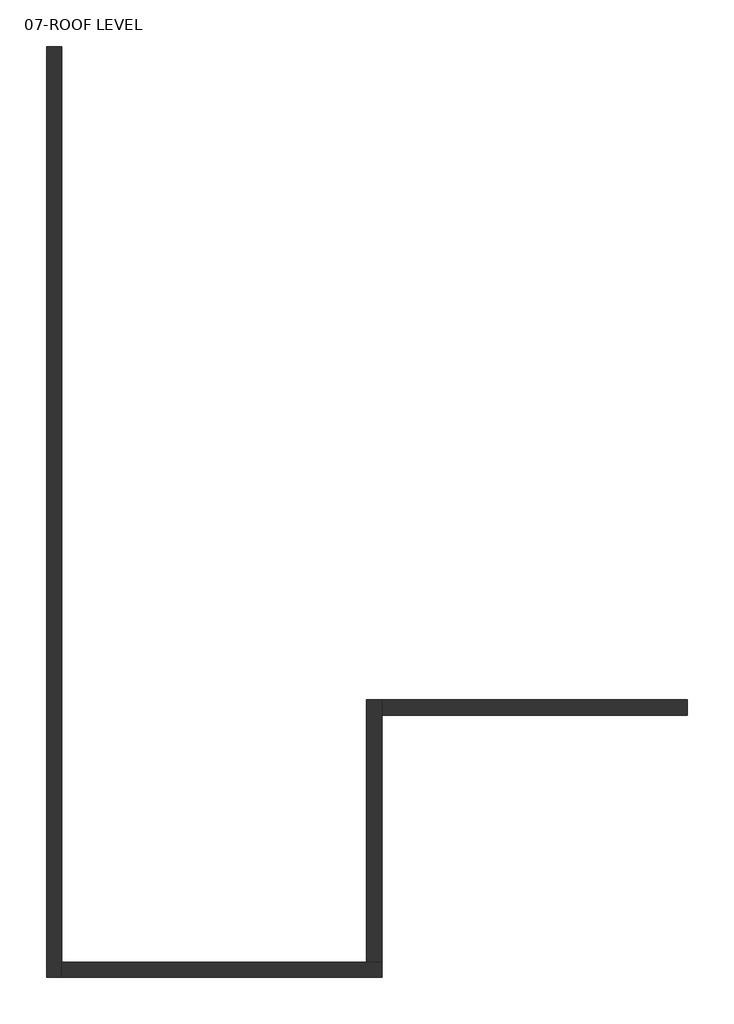
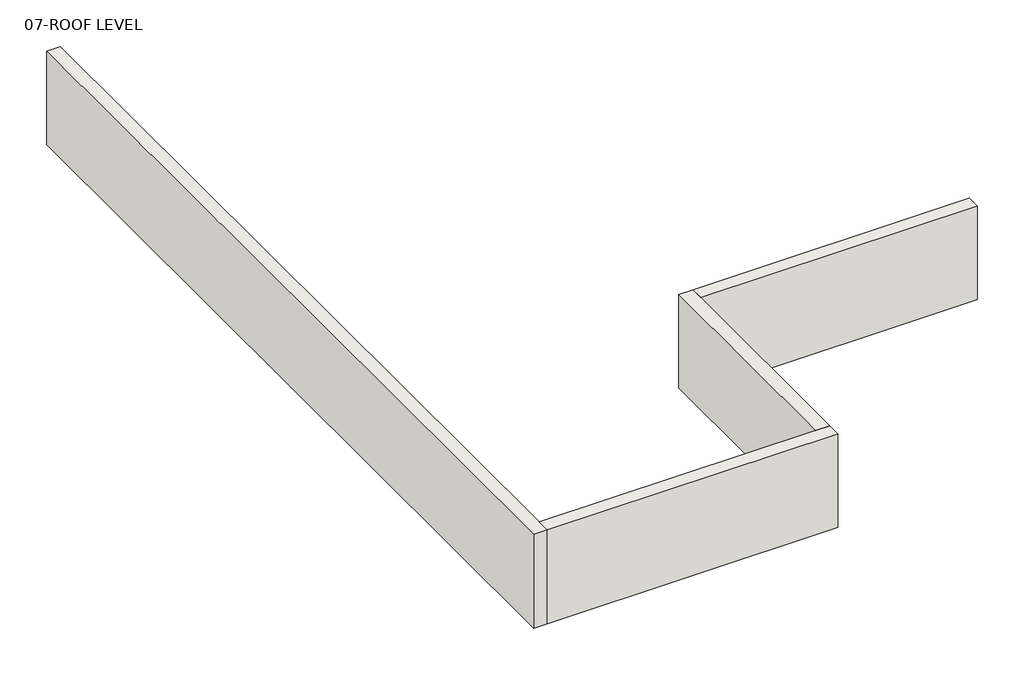
# One storey: 4 walls.
"""IFC4 building model written with IfcOpenShell, lengths in millimetres."""

from ifc_helpers import new_model, si_unit, frame, origin, place, context, project, spatial, polyline, outline, extrude, faceted_brep, element, save

model = new_model("IFC4")

# Units and contexts
model_context = context("Model", 3, world=origin())
ifc_project = project(units=[si_unit("LENGTHUNIT", "METRE", prefix="MILLI")], contexts=[model_context])

# Site, building, storey
site = spatial("IfcSite", under=ifc_project)
building = spatial("IfcBuilding", under=site)
storey = spatial("IfcBuildingStorey", under=building, Name="07-ROOF LEVEL", Elevation=7350.0)

# Walls
placement = place(None, origin())
element("IfcWall", 1, ObjectType="01-225 WALL MAIN", at=placement, inside=storey, context=model_context, shape_type="Brep", body=[
    faceted_brep([(-14560.1792561, 6713.2802318, 7350.0), (-14560.1792561, -6069.2197682, 7350.0), (-14560.1792561, -6069.2197682, 8850.0), (-14560.1792561, 6713.2802318, 8850.0), (-14350.1792561, 6713.2802318, 7350.0), (-14350.1792561, 6713.2802318, 8850.0), (-14350.1792561, -5859.2197682, 8850.0), (-14350.1792561, -6069.2197682, 8850.0), (-14350.1792561, -6069.2197682, 7350.0), (-14350.1792561, -5859.2197682, 7350.0)], [[[0, 1, 2, 3]], [[4, 5, 6, 7, 8, 9]], [[1, 0, 4, 9, 8]], [[3, 2, 7, 6, 5]], [[0, 3, 5, 4]], [[2, 1, 8, 7]]]),
])
element("IfcWall", 2, ObjectType="01-225 WALL MAIN", at=placement, inside=storey, context=model_context, shape_type="Brep", body=[
    faceted_brep([(-14350.1792561, -6069.2197682, 7350.0), (-9950.1792561, -6069.2197682, 7350.0), (-9950.1792561, -6069.2197682, 8850.0), (-14350.1792561, -6069.2197682, 8850.0), (-14350.1792561, -5859.2197682, 7350.0), (-14350.1792561, -5859.2197682, 8850.0), (-10160.1792561, -5859.2197682, 8850.0), (-9950.1792561, -5859.2197682, 8850.0), (-9950.1792561, -5859.2197682, 7350.0), (-10160.1792561, -5859.2197682, 7350.0)], [[[0, 1, 2, 3]], [[4, 5, 6, 7, 8, 9]], [[1, 0, 4, 9, 8]], [[3, 2, 7, 6, 5]], [[0, 3, 5, 4]], [[2, 1, 8, 7]]]),
])
element("IfcWall", 3, ObjectType="01-225 WALL MAIN", at=placement, inside=storey, context=model_context, shape_type="Brep", body=[
    faceted_brep([(-9950.1792561, -5859.2197682, 7350.0), (-9950.1792561, -2469.2197682, 7350.0), (-9950.1792561, -2259.2197682, 7350.0), (-9950.1792561, -2259.2197682, 8850.0), (-9950.1792561, -2469.2197682, 8850.0), (-9950.1792561, -5859.2197682, 8850.0), (-10160.1792561, -5859.2197682, 7350.0), (-10160.1792561, -5859.2197682, 8850.0), (-10160.1792561, -2259.2197682, 8850.0), (-10160.1792561, -2259.2197682, 7350.0)], [[[0, 1, 2, 3, 4, 5]], [[6, 7, 8, 9]], [[2, 1, 0, 6, 9]], [[5, 4, 3, 8, 7]], [[0, 5, 7, 6]], [[3, 2, 9, 8]]]),
])
element("IfcWall", 4, ObjectType="01-225 WALL MAIN", at=placement, inside=storey, context=model_context, shape_type="SweptSolid", body=[
    extrude(outline(polyline([(-5755.1792561, -2469.2197682), (-9950.1792561, -2469.2197682), (-9950.1792561, -2259.2197682), (-5755.1792561, -2259.2197682), (-5755.1792561, -2469.2197682)])), frame((0.0, 0.0, 7350.0), z_axis=(0.0, 0.0, 1.0), x_axis=(1.0, 0.0, 0.0)), (0.0, 0.0, 1.0), 1500.0),
])

save(model, "model.ifc")

# Revit data of these elements
# Type "01-225 WALL MAIN"
#   Description = "Generic Wall (Material By Category), 200mm thick"
#   Assembly Code = "B2010"
#   Type Mark = "G06"
#   Layers, outside or top first: 5 mm "01-WHITE WALL PAINT" (function 4); 200 mm "01-DEFAULT WALL" (function 1); 5 mm "01-WHITE WALL PAINT" (function 5)
# Elements 1, 2, 3 (IfcWall, "01-225 WALL MAIN")
#   Top Offset = 0 mm
#   Base Offset = 0 mm
#   wall height = 1500 mm
#   Phase Created = New Construction
#   Base Constraint = 07-ROOF LEVEL
#   Top Constraint = 08-PARAPET LEVEL
#   Materials on its faces: "01-WHITE WALL PAINT", "Default Wall"
# Element 4 (IfcWall, "01-225 WALL MAIN")
#   Top Offset = 0 mm
#   Base Offset = 0 mm
#   wall height = 1500 mm
#   Phase Created = New Construction
#   Base Constraint = 07-ROOF LEVEL
#   Top Constraint = 08-PARAPET LEVEL
#   Materials on its faces: "Default Wall", "01-WHITE WALL PAINT"
# Materials
#   "01-WHITE WALL PAINT": class "Generic", colour RGB 242 242 255, transparency 0, Description = "Acoustic Ceiling Tile 24 x 48", Cost = 0
#   "01-DEFAULT WALL": class "Generic", colour RGB 242 242 255, transparency 0, Description = "Acoustic Ceiling Tile 24 x 48", Cost = 0
#   "Default Wall": colour RGB 192 192 192, transparency 0, Cost = 0
